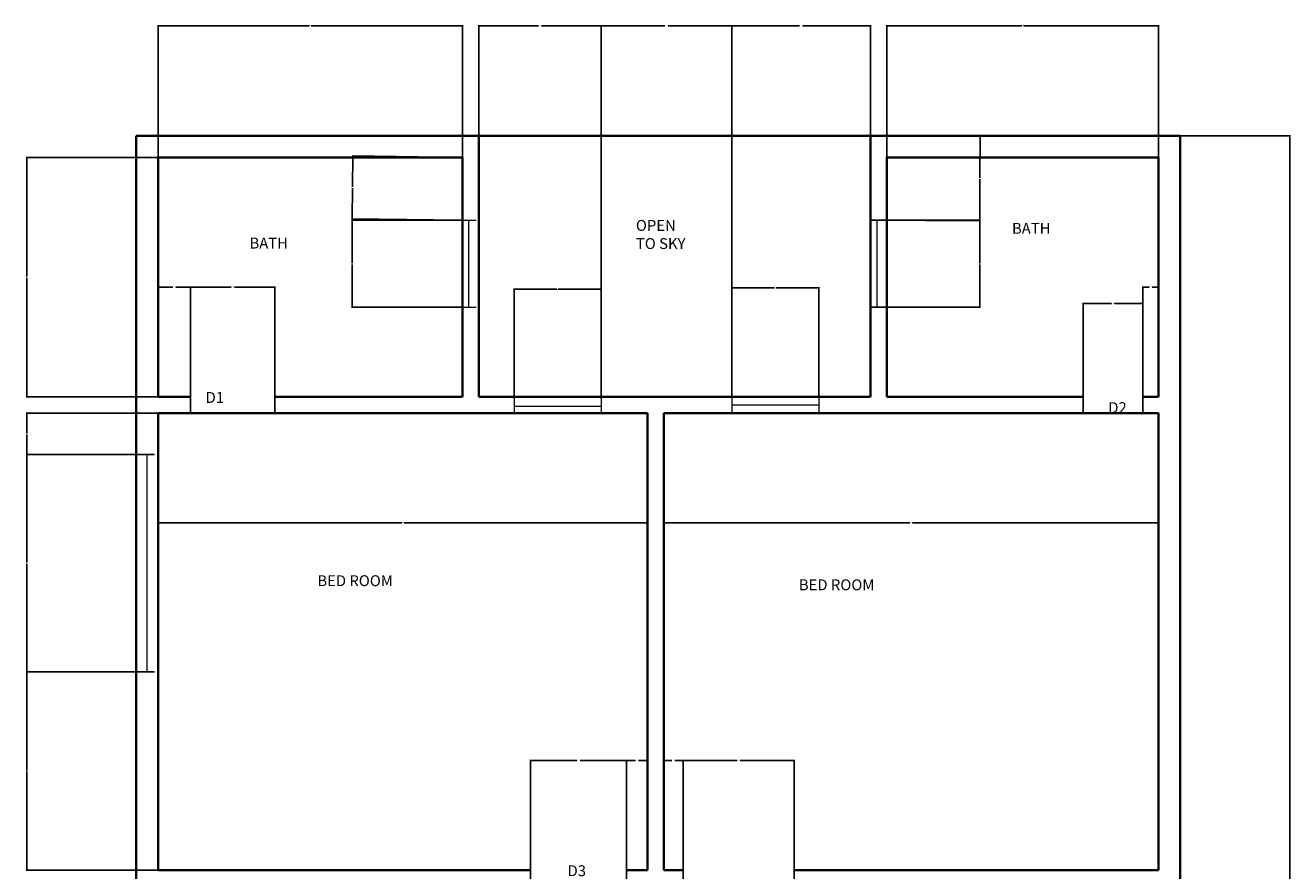
# Model space of a CAD drawing. Units: inches. Extents: x 301 to 1174, y -458 to 167.
# Tile 4 of 4: x 825 to 1174, y -66 to 167. Entities that reach past the tile are written whole.
import ezdxf

# ---------------------------------------------------------------- set-up
doc = ezdxf.new("R2010")
doc.units = ezdxf.units.IN
doc.header["$MEASUREMENT"] = 0
for name, color, linetype, lineweight in [('A-ANNO-DIMS', 2, 'Continuous', 18), ('A-ANNO-TEXT', 7, 'Continuous', 25), ('A-AREA-IDEN', 7, 'Continuous', 18), ('A-DOOR', 3, 'Continuous', 25), ('A-GLAZ', 4, 'Continuous', 18), ('A-WALL', 7, 'Continuous', 35)]:
    doc.layers.add(name, color=color, linetype=linetype, lineweight=lineweight)
doc.styles.get("Standard").update_dxf_attribs({"font": 'arial.ttf'})
doc.dimstyles.get("Standard").update_dxf_attribs({"dimtxt": 0.18, "dimasz": 0.18, "dimexe": 0.18, "dimexo": 0.0625, "dimgap": 0.09, "dimtad": 0, "dimtih": 1, "dimtoh": 1, "dimdec": 4, "dimzin": 0, "dimdsep": 46, "dimtxsty": 'Standard', "dimcen": 0.09, "dimadec": 0, "dimazin": 0, "dimtfac": 1, "dimtdec": 4, "dimtofl": 0, "dimtmove": 0, "dimatfit": 3, "dimfxl": 1, "dimtolj": 1, "dimtzin": 0, "dimarcsym": 0})

# ---------------------------------------------------------------- blocks, each defined once
blk = doc.blocks.new('*U2')
for p, q in [((0, 4), (0, 0)), ((24, 4), (24, 0)), ((0, 2), (24, 2))]:
    blk.add_line(p, q)
blk = doc.blocks.new('*U4')
for p, q in [((0, 4), (0, 0)), ((60, 4), (60, 0)), ((0, 2), (60, 2))]:
    blk.add_line(p, q)
blk = doc.blocks.new('*D39')
at = {"layer": 'A-ANNO-DIMS', "color": 0, "lineweight": -2, "transparency": 16777216}
for p, q in [((1143.26, 136.8), (1173.63, 136.8)), ((1173.45, 136.62), (1173.45, -133.02)), ((1173.45, -403.02), (1173.45, -133.38)), ((1143.26, -403.2), (1173.63, -403.2))]:
    blk.add_line(p, q, dxfattribs=at)
at = {"layer": 'A-ANNO-DIMS', "color": 0, "transparency": 16777216}
for points in [[(1173.42, 136.62), (1173.48, 136.62), (1173.45, 136.8)], [(1173.42, -403.02), (1173.48, -403.02), (1173.45, -403.2)]]:
    blk.add_solid(points, dxfattribs=at)
at = {"layer": 'Defpoints', "color": 0, "transparency": 16777216}
for p in [(1143.2, 136.8), (1173.45, 136.8), (1143.2, -403.2)]:
    blk.add_point(p, dxfattribs=at)
at = {"layer": 'A-ANNO-DIMS', "color": 0, "transparency": 16777216, "insert": (1173.45, -133.2), "char_height": 0.18, "attachment_point": 5}
blk.add_mtext('\\A1;540', dxfattribs=at)
blk = doc.blocks.new('*D40')
at = {"layer": 'A-ANNO-DIMS', "color": 0, "lineweight": -2, "transparency": 16777216}
for p, q in [((861.2, 130.86), (861.2, 167.23)), ((861.38, 167.05), (902.98, 167.05)), ((945.02, 167.05), (903.42, 167.05)), ((945.2, 130.86), (945.2, 167.23))]:
    blk.add_line(p, q, dxfattribs=at)
at = {"layer": 'A-ANNO-DIMS', "color": 0, "transparency": 16777216}
for points in [[(861.38, 167.08), (861.38, 167.02), (861.2, 167.05)], [(945.02, 167.08), (945.02, 167.02), (945.2, 167.05)]]:
    blk.add_solid(points, dxfattribs=at)
at = {"layer": 'Defpoints', "color": 0, "transparency": 16777216}
for p in [(945.2, 167.05), (861.2, 130.8), (945.2, 130.8)]:
    blk.add_point(p, dxfattribs=at)
at = {"layer": 'A-ANNO-DIMS', "color": 0, "transparency": 16777216, "insert": (903.2, 167.05), "char_height": 0.18, "attachment_point": 5}
blk.add_mtext('\\A1;84', dxfattribs=at)
blk = doc.blocks.new('*D41')
at = {"layer": 'A-ANNO-DIMS', "color": 0, "lineweight": -2, "transparency": 16777216}
for p, q in [((949.7, 136.86), (949.7, 167.23)), ((949.88, 167.05), (966.15, 167.05)), ((983.21, 167.05), (966.94, 167.05)), ((983.39, 64.27), (983.39, 167.23))]:
    blk.add_line(p, q, dxfattribs=at)
at = {"layer": 'A-ANNO-DIMS', "color": 0, "transparency": 16777216}
for points in [[(949.88, 167.08), (949.88, 167.02), (949.7, 167.05)], [(983.21, 167.08), (983.21, 167.02), (983.39, 167.05)]]:
    blk.add_solid(points, dxfattribs=at)
at = {"layer": 'Defpoints', "color": 0, "transparency": 16777216}
for p in [(983.39, 167.05), (949.7, 136.8), (983.39, 64.21)]:
    blk.add_point(p, dxfattribs=at)
at = {"layer": 'A-ANNO-DIMS', "color": 0, "transparency": 16777216, "insert": (966.54, 167.05), "char_height": 0.18, "attachment_point": 5}
blk.add_mtext('\\A1;33.69', dxfattribs=at)
blk = doc.blocks.new('*D42')
at = {"layer": 'A-ANNO-DIMS', "color": 0, "lineweight": -2, "transparency": 16777216}
for p, q in [((983.39, 64.27), (983.39, 167.23)), ((983.57, 167.05), (1000.97, 167.05)), ((1019.29, 167.05), (1001.89, 167.05)), ((1019.47, 64.65), (1019.47, 167.23))]:
    blk.add_line(p, q, dxfattribs=at)
at = {"layer": 'A-ANNO-DIMS', "color": 0, "transparency": 16777216}
for points in [[(983.57, 167.08), (983.57, 167.02), (983.39, 167.05)], [(1019.29, 167.08), (1019.29, 167.02), (1019.47, 167.05)]]:
    blk.add_solid(points, dxfattribs=at)
at = {"layer": 'Defpoints', "color": 0, "transparency": 16777216}
for p in [(1019.47, 167.05), (983.39, 64.21), (1019.47, 64.59)]:
    blk.add_point(p, dxfattribs=at)
at = {"layer": 'A-ANNO-DIMS', "color": 0, "transparency": 16777216, "insert": (1001.43, 167.05), "char_height": 0.18, "attachment_point": 5}
blk.add_mtext('\\A1;36.086', dxfattribs=at)
blk = doc.blocks.new('*D43')
at = {"layer": 'A-ANNO-DIMS', "color": 0, "lineweight": -2, "transparency": 16777216}
for p, q in [((1019.47, 64.65), (1019.47, 167.23)), ((1019.65, 167.05), (1038.19, 167.05)), ((1057.52, 167.05), (1038.98, 167.05)), ((1057.7, 136.86), (1057.7, 167.23))]:
    blk.add_line(p, q, dxfattribs=at)
at = {"layer": 'A-ANNO-DIMS', "color": 0, "transparency": 16777216}
for points in [[(1019.65, 167.08), (1019.65, 167.02), (1019.47, 167.05)], [(1057.52, 167.08), (1057.52, 167.02), (1057.7, 167.05)]]:
    blk.add_solid(points, dxfattribs=at)
at = {"layer": 'Defpoints', "color": 0, "transparency": 16777216}
for p in [(1057.7, 167.05), (1057.7, 136.8), (1019.47, 64.59)]:
    blk.add_point(p, dxfattribs=at)
at = {"layer": 'A-ANNO-DIMS', "color": 0, "transparency": 16777216, "insert": (1038.59, 167.05), "char_height": 0.18, "attachment_point": 5}
blk.add_mtext('\\A1;38.22', dxfattribs=at)
blk = doc.blocks.new('*D44')
at = {"layer": 'A-ANNO-DIMS', "color": 0, "lineweight": -2, "transparency": 16777216}
for p, q in [((1062.2, 130.86), (1062.2, 167.23)), ((1062.38, 167.05), (1099.48, 167.05)), ((1137.02, 167.05), (1099.92, 167.05)), ((1137.2, 130.86), (1137.2, 167.23))]:
    blk.add_line(p, q, dxfattribs=at)
at = {"layer": 'A-ANNO-DIMS', "color": 0, "transparency": 16777216}
for points in [[(1062.38, 167.08), (1062.38, 167.02), (1062.2, 167.05)], [(1137.02, 167.08), (1137.02, 167.02), (1137.2, 167.05)]]:
    blk.add_solid(points, dxfattribs=at)
at = {"layer": 'Defpoints', "color": 0, "transparency": 16777216}
for p in [(1137.2, 167.05), (1062.2, 130.8), (1137.2, 130.8)]:
    blk.add_point(p, dxfattribs=at)
at = {"layer": 'A-ANNO-DIMS', "color": 0, "transparency": 16777216, "insert": (1099.7, 167.05), "char_height": 0.18, "attachment_point": 5}
blk.add_mtext('\\A1;75', dxfattribs=at)
blk = doc.blocks.new('*D45')
at = {"layer": 'A-ANNO-DIMS', "color": 0, "lineweight": -2, "transparency": 16777216}
for p, q in [((959.39, 64.27), (959.39, 94.64)), ((959.57, 94.46), (971.17, 94.46)), ((983.21, 94.46), (971.61, 94.46)), ((983.39, 64.27), (983.39, 94.64))]:
    blk.add_line(p, q, dxfattribs=at)
at = {"layer": 'A-ANNO-DIMS', "color": 0, "transparency": 16777216}
for points in [[(959.57, 94.49), (959.57, 94.43), (959.39, 94.46)], [(983.21, 94.49), (983.21, 94.43), (983.39, 94.46)]]:
    blk.add_solid(points, dxfattribs=at)
at = {"layer": 'Defpoints', "color": 0, "transparency": 16777216}
for p in [(983.39, 94.46), (959.39, 64.21), (983.39, 64.21)]:
    blk.add_point(p, dxfattribs=at)
at = {"layer": 'A-ANNO-DIMS', "color": 0, "transparency": 16777216, "insert": (971.39, 94.46), "char_height": 0.18, "attachment_point": 5}
blk.add_mtext('\\A1;24', dxfattribs=at)
blk = doc.blocks.new('*D46')
at = {"layer": 'A-ANNO-DIMS', "color": 0, "lineweight": -2, "transparency": 16777216}
for p, q in [((1019.47, 64.65), (1019.47, 95.02)), ((1019.65, 94.84), (1031.25, 94.84)), ((1043.29, 94.84), (1031.69, 94.84)), ((1043.47, 64.65), (1043.47, 95.02))]:
    blk.add_line(p, q, dxfattribs=at)
at = {"layer": 'A-ANNO-DIMS', "color": 0, "transparency": 16777216}
for points in [[(1019.65, 94.87), (1019.65, 94.81), (1019.47, 94.84)], [(1043.29, 94.87), (1043.29, 94.81), (1043.47, 94.84)]]:
    blk.add_solid(points, dxfattribs=at)
at = {"layer": 'Defpoints', "color": 0, "transparency": 16777216}
for p in [(1043.47, 94.84), (1019.47, 64.59), (1043.47, 64.59)]:
    blk.add_point(p, dxfattribs=at)
at = {"layer": 'A-ANNO-DIMS', "color": 0, "transparency": 16777216, "insert": (1031.47, 94.84), "char_height": 0.18, "attachment_point": 5}
blk.add_mtext('\\A1;24', dxfattribs=at)
blk = doc.blocks.new('*D47')
at = {"layer": 'A-ANNO-DIMS', "color": 0, "lineweight": -2, "transparency": 16777216}
for p, q in [((861.2, 60.24), (861.2, 29.87)), ((996.2, 60.24), (996.2, 29.87)), ((861.38, 30.05), (928.42, 30.05)), ((996.02, 30.05), (928.98, 30.05))]:
    blk.add_line(p, q, dxfattribs=at)
at = {"layer": 'A-ANNO-DIMS', "color": 0, "transparency": 16777216}
for points in [[(861.38, 30.08), (861.38, 30.02), (861.2, 30.05)], [(996.02, 30.08), (996.02, 30.02), (996.2, 30.05)]]:
    blk.add_solid(points, dxfattribs=at)
at = {"layer": 'Defpoints', "color": 0, "transparency": 16777216}
for p in [(861.2, 60.3), (996.2, 60.3), (861.2, 30.05)]:
    blk.add_point(p, dxfattribs=at)
at = {"layer": 'A-ANNO-DIMS', "color": 0, "transparency": 16777216, "insert": (928.7, 30.05), "char_height": 0.18, "attachment_point": 5}
blk.add_mtext('\\A1;135', dxfattribs=at)
blk = doc.blocks.new('*D48')
at = {"layer": 'A-ANNO-DIMS', "color": 0, "lineweight": -2, "transparency": 16777216}
for p, q in [((1000.7, 60.24), (1000.7, 29.87)), ((1137.2, 60.24), (1137.2, 29.87)), ((1000.88, 30.05), (1068.56, 30.05)), ((1137.02, 30.05), (1069.33, 30.05))]:
    blk.add_line(p, q, dxfattribs=at)
at = {"layer": 'A-ANNO-DIMS', "color": 0, "transparency": 16777216}
for points in [[(1000.88, 30.08), (1000.88, 30.02), (1000.7, 30.05)], [(1137.02, 30.08), (1137.02, 30.02), (1137.2, 30.05)]]:
    blk.add_solid(points, dxfattribs=at)
at = {"layer": 'Defpoints', "color": 0, "transparency": 16777216}
for p in [(1000.7, 60.3), (1137.2, 60.3), (1000.7, 30.05)]:
    blk.add_point(p, dxfattribs=at)
at = {"layer": 'A-ANNO-DIMS', "color": 0, "transparency": 16777216, "insert": (1068.95, 30.05), "char_height": 0.18, "attachment_point": 5}
blk.add_mtext('\\A1;136.5', dxfattribs=at)
blk = doc.blocks.new('*D55')
at = {"layer": 'A-ANNO-DIMS', "color": 0, "lineweight": -2, "transparency": 16777216}
for p, q in [((861.13, 130.8), (824.77, 130.8)), ((824.95, 130.62), (824.95, 97.98)), ((824.95, 64.98), (824.95, 97.62)), ((861.13, 64.8), (824.77, 64.8))]:
    blk.add_line(p, q, dxfattribs=at)
at = {"layer": 'A-ANNO-DIMS', "color": 0, "transparency": 16777216}
for points in [[(824.92, 130.62), (824.98, 130.62), (824.95, 130.8)], [(824.92, 64.98), (824.98, 64.98), (824.95, 64.8)]]:
    blk.add_solid(points, dxfattribs=at)
at = {"layer": 'Defpoints', "color": 0, "transparency": 16777216}
for p in [(824.95, 130.8), (861.2, 130.8), (861.2, 64.8)]:
    blk.add_point(p, dxfattribs=at)
at = {"layer": 'A-ANNO-DIMS', "color": 0, "transparency": 16777216, "insert": (824.95, 97.8), "char_height": 0.18, "attachment_point": 5}
blk.add_mtext('\\A1;66', dxfattribs=at)
blk = doc.blocks.new('*D56')
at = {"layer": 'A-ANNO-DIMS', "color": 0, "lineweight": -2, "transparency": 16777216}
for p, q in [((860.11, -11.08), (824.77, -11.08)), ((824.95, -11.26), (824.95, -38.21)), ((824.95, -65.52), (824.95, -38.57)), ((861.13, -65.7), (824.77, -65.7))]:
    blk.add_line(p, q, dxfattribs=at)
at = {"layer": 'A-ANNO-DIMS', "color": 0, "transparency": 16777216}
for points in [[(824.92, -11.26), (824.98, -11.26), (824.95, -11.08)], [(824.92, -65.52), (824.98, -65.52), (824.95, -65.7)]]:
    blk.add_solid(points, dxfattribs=at)
at = {"layer": 'Defpoints', "color": 0, "transparency": 16777216}
for p in [(824.95, -11.08), (860.17, -11.08), (861.2, -65.7)]:
    blk.add_point(p, dxfattribs=at)
at = {"layer": 'A-ANNO-DIMS', "color": 0, "transparency": 16777216, "insert": (824.95, -38.39), "char_height": 0.18, "attachment_point": 5}
blk.add_mtext('\\A1;54.61', dxfattribs=at)
blk = doc.blocks.new('*D57')
at = {"layer": 'A-ANNO-DIMS', "color": 0, "lineweight": -2, "transparency": 16777216}
for p, q in [((860.11, 48.92), (824.77, 48.92)), ((824.95, 48.74), (824.95, 19.1)), ((824.95, -10.9), (824.95, 18.73)), ((860.11, -11.08), (824.77, -11.08))]:
    blk.add_line(p, q, dxfattribs=at)
at = {"layer": 'A-ANNO-DIMS', "color": 0, "transparency": 16777216}
for points in [[(824.92, 48.74), (824.98, 48.74), (824.95, 48.92)], [(824.92, -10.9), (824.98, -10.9), (824.95, -11.08)]]:
    blk.add_solid(points, dxfattribs=at)
at = {"layer": 'Defpoints', "color": 0, "transparency": 16777216}
for p in [(824.95, 48.92), (860.17, 48.92), (860.17, -11.08)]:
    blk.add_point(p, dxfattribs=at)
at = {"layer": 'A-ANNO-DIMS', "color": 0, "transparency": 16777216, "insert": (824.95, 18.92), "char_height": 0.18, "attachment_point": 5}
blk.add_mtext('\\A1;60', dxfattribs=at)
blk = doc.blocks.new('*D58')
at = {"layer": 'A-ANNO-DIMS', "color": 0, "lineweight": -2, "transparency": 16777216}
for p, q in [((861.13, 60.3), (824.77, 60.3)), ((824.95, 60.12), (824.95, 54.79)), ((824.95, 49.1), (824.95, 54.43)), ((860.11, 48.92), (824.77, 48.92))]:
    blk.add_line(p, q, dxfattribs=at)
at = {"layer": 'A-ANNO-DIMS', "color": 0, "transparency": 16777216}
for points in [[(824.92, 60.12), (824.98, 60.12), (824.95, 60.3)], [(824.92, 49.1), (824.98, 49.1), (824.95, 48.92)]]:
    blk.add_solid(points, dxfattribs=at)
at = {"layer": 'Defpoints', "color": 0, "transparency": 16777216}
for p in [(824.95, 60.3), (861.2, 60.3), (860.17, 48.92)]:
    blk.add_point(p, dxfattribs=at)
at = {"layer": 'A-ANNO-DIMS', "color": 0, "transparency": 16777216, "insert": (824.95, 54.61), "char_height": 0.18, "attachment_point": 5}
blk.add_mtext('\\A1;11.386', dxfattribs=at)
blk = doc.blocks.new('*D66')
at = {"layer": 'A-ANNO-DIMS', "color": 0, "lineweight": -2, "transparency": 16777216}
for p, q in [((861.2, 64.86), (861.2, 95.23)), ((861.38, 95.05), (865.29, 95.05)), ((869.98, 95.05), (866.07, 95.05)), ((870.16, 64.86), (870.16, 95.23))]:
    blk.add_line(p, q, dxfattribs=at)
at = {"layer": 'A-ANNO-DIMS', "color": 0, "transparency": 16777216}
for points in [[(861.38, 95.08), (861.38, 95.02), (861.2, 95.05)], [(869.98, 95.08), (869.98, 95.02), (870.16, 95.05)]]:
    blk.add_solid(points, dxfattribs=at)
at = {"layer": 'Defpoints', "color": 0, "transparency": 16777216}
for p in [(870.16, 95.05), (861.2, 64.8), (870.16, 64.8)]:
    blk.add_point(p, dxfattribs=at)
at = {"layer": 'A-ANNO-DIMS', "color": 0, "transparency": 16777216, "insert": (865.68, 95.05), "char_height": 0.18, "attachment_point": 5}
blk.add_mtext('\\A1;8.962', dxfattribs=at)
blk = doc.blocks.new('*D67')
at = {"layer": 'A-ANNO-DIMS', "color": 0, "lineweight": -2, "transparency": 16777216}
for p, q in [((870.16, 64.86), (870.16, 95.23)), ((870.34, 95.05), (881.33, 95.05)), ((893.25, 95.05), (882.26, 95.05)), ((893.43, 64.86), (893.43, 95.23))]:
    blk.add_line(p, q, dxfattribs=at)
at = {"layer": 'A-ANNO-DIMS', "color": 0, "transparency": 16777216}
for points in [[(870.34, 95.08), (870.34, 95.02), (870.16, 95.05)], [(893.25, 95.08), (893.25, 95.02), (893.43, 95.05)]]:
    blk.add_solid(points, dxfattribs=at)
at = {"layer": 'Defpoints', "color": 0, "transparency": 16777216}
for p in [(893.43, 95.05), (870.16, 64.8), (893.43, 64.8)]:
    blk.add_point(p, dxfattribs=at)
at = {"layer": 'A-ANNO-DIMS', "color": 0, "transparency": 16777216, "insert": (881.79, 95.05), "char_height": 0.18, "attachment_point": 5}
blk.add_mtext('\\A1;23.267', dxfattribs=at)
blk = doc.blocks.new('*D68')
at = {"layer": 'A-ANNO-DIMS', "color": 0, "lineweight": -2, "transparency": 16777216}
for p, q in [((1116.42, 60.36), (1116.42, 90.73)), ((1116.6, 90.55), (1124.18, 90.55)), ((1132.68, 90.55), (1125.09, 90.55)), ((1132.86, 60.36), (1132.86, 90.73))]:
    blk.add_line(p, q, dxfattribs=at)
at = {"layer": 'A-ANNO-DIMS', "color": 0, "transparency": 16777216}
for points in [[(1116.6, 90.58), (1116.6, 90.52), (1116.42, 90.55)], [(1132.68, 90.58), (1132.68, 90.52), (1132.86, 90.55)]]:
    blk.add_solid(points, dxfattribs=at)
at = {"layer": 'Defpoints', "color": 0, "transparency": 16777216}
for p in [(1132.86, 90.55), (1116.42, 60.3), (1132.86, 60.3)]:
    blk.add_point(p, dxfattribs=at)
at = {"layer": 'A-ANNO-DIMS', "color": 0, "transparency": 16777216, "insert": (1124.64, 90.55), "char_height": 0.18, "attachment_point": 5}
blk.add_mtext('\\A1;16.434', dxfattribs=at)
blk = doc.blocks.new('*D69')
at = {"layer": 'A-ANNO-DIMS', "color": 0, "lineweight": -2, "transparency": 16777216}
for p, q in [((1132.86, 64.86), (1132.86, 95.23)), ((1133.04, 95.05), (1134.63, 95.05)), ((1137.02, 95.05), (1135.42, 95.05)), ((1137.2, 64.86), (1137.2, 95.23))]:
    blk.add_line(p, q, dxfattribs=at)
at = {"layer": 'A-ANNO-DIMS', "color": 0, "transparency": 16777216}
for points in [[(1133.04, 95.08), (1133.04, 95.02), (1132.86, 95.05)], [(1137.02, 95.08), (1137.02, 95.02), (1137.2, 95.05)]]:
    blk.add_solid(points, dxfattribs=at)
at = {"layer": 'Defpoints', "color": 0, "transparency": 16777216}
for p in [(1137.2, 95.05), (1132.86, 64.8), (1137.2, 64.8)]:
    blk.add_point(p, dxfattribs=at)
at = {"layer": 'A-ANNO-DIMS', "color": 0, "transparency": 16777216, "insert": (1135.03, 95.05), "char_height": 0.18, "attachment_point": 5}
blk.add_mtext('\\A1;4.342', dxfattribs=at)
blk = doc.blocks.new('*D70')
at = {"layer": 'A-ANNO-DIMS', "color": 0, "lineweight": -2, "transparency": 16777216}
for p, q in [((944.9, 113.47), (914.54, 113.47)), ((914.72, 113.29), (914.72, 101.65)), ((914.72, 89.65), (914.72, 101.29)), ((944.9, 89.47), (914.54, 89.47))]:
    blk.add_line(p, q, dxfattribs=at)
at = {"layer": 'A-ANNO-DIMS', "color": 0, "transparency": 16777216}
for points in [[(914.69, 113.29), (914.75, 113.29), (914.72, 113.47)], [(914.69, 89.65), (914.75, 89.65), (914.72, 89.47)]]:
    blk.add_solid(points, dxfattribs=at)
at = {"layer": 'Defpoints', "color": 0, "transparency": 16777216}
for p in [(914.72, 113.47), (944.97, 113.47), (944.97, 89.47)]:
    blk.add_point(p, dxfattribs=at)
at = {"layer": 'A-ANNO-DIMS', "color": 0, "transparency": 16777216, "insert": (914.72, 101.47), "char_height": 0.18, "attachment_point": 5}
blk.add_mtext('\\A1;24', dxfattribs=at)
blk = doc.blocks.new('*D71')
at = {"layer": 'A-ANNO-DIMS', "color": 0, "lineweight": -2, "transparency": 16777216}
for p, q in [((945.13, 130.8), (914.77, 131.21)), ((914.95, 131.02), (914.84, 122.72)), ((914.72, 114.05), (914.83, 122.36)), ((944.9, 113.47), (914.54, 113.87))]:
    blk.add_line(p, q, dxfattribs=at)
at = {"layer": 'A-ANNO-DIMS', "color": 0, "transparency": 16777216}
for points in [[(914.92, 131.02), (914.98, 131.02), (914.95, 131.2)], [(914.69, 114.05), (914.75, 114.05), (914.72, 113.87)]]:
    blk.add_solid(points, dxfattribs=at)
at = {"layer": 'Defpoints', "color": 0, "transparency": 16777216}
for p in [(914.95, 131.2), (945.2, 130.8), (944.97, 113.47)]:
    blk.add_point(p, dxfattribs=at)
at = {"layer": 'A-ANNO-DIMS', "color": 0, "transparency": 16777216, "insert": (914.83, 122.54), "char_height": 0.18, "attachment_point": 5}
blk.add_mtext('\\A1;17.334', dxfattribs=at)
blk = doc.blocks.new('*D72')
at = {"layer": 'A-ANNO-DIMS', "color": 0, "lineweight": -2, "transparency": 16777216}
for p, q in [((1057.76, 136.8), (1088.13, 136.69)), ((1087.95, 136.51), (1087.9, 125.2)), ((1087.86, 113.54), (1087.9, 124.84)), ((1057.67, 113.47), (1088.04, 113.36))]:
    blk.add_line(p, q, dxfattribs=at)
at = {"layer": 'A-ANNO-DIMS', "color": 0, "transparency": 16777216}
for points in [[(1087.92, 136.51), (1087.98, 136.51), (1087.95, 136.69)], [(1087.83, 113.54), (1087.89, 113.54), (1087.86, 113.36)]]:
    blk.add_solid(points, dxfattribs=at)
at = {"layer": 'Defpoints', "color": 0, "transparency": 16777216}
for p in [(1057.7, 136.8), (1057.61, 113.47), (1087.86, 113.36)]:
    blk.add_point(p, dxfattribs=at)
at = {"layer": 'A-ANNO-DIMS', "color": 0, "transparency": 16777216, "insert": (1087.9, 125.02), "char_height": 0.18, "attachment_point": 5}
blk.add_mtext('\\A1;23.33', dxfattribs=at)
blk = doc.blocks.new('*D73')
at = {"layer": 'A-ANNO-DIMS', "color": 0, "lineweight": -2, "transparency": 16777216}
for p, q in [((1057.67, 113.47), (1088.04, 113.47)), ((1087.86, 113.29), (1087.86, 101.65)), ((1087.86, 89.65), (1087.86, 101.29)), ((1057.67, 89.47), (1088.04, 89.47))]:
    blk.add_line(p, q, dxfattribs=at)
at = {"layer": 'A-ANNO-DIMS', "color": 0, "transparency": 16777216}
for points in [[(1087.83, 113.29), (1087.89, 113.29), (1087.86, 113.47)], [(1087.83, 89.65), (1087.89, 89.65), (1087.86, 89.47)]]:
    blk.add_solid(points, dxfattribs=at)
at = {"layer": 'Defpoints', "color": 0, "transparency": 16777216}
for p in [(1057.61, 113.47), (1057.61, 89.47), (1087.86, 89.47)]:
    blk.add_point(p, dxfattribs=at)
at = {"layer": 'A-ANNO-DIMS', "color": 0, "transparency": 16777216, "insert": (1087.86, 101.47), "char_height": 0.18, "attachment_point": 5}
blk.add_mtext('\\A1;24', dxfattribs=at)
blk = doc.blocks.new('*D74')
at = {"layer": 'A-ANNO-DIMS', "color": 0, "lineweight": -2, "transparency": 16777216}
for p, q in [((963.97, -65.64), (963.97, -35.27)), ((964.15, -35.45), (976.74, -35.45)), ((990.26, -35.45), (977.67, -35.45)), ((990.44, -65.64), (990.44, -35.27))]:
    blk.add_line(p, q, dxfattribs=at)
at = {"layer": 'A-ANNO-DIMS', "color": 0, "transparency": 16777216}
for points in [[(964.15, -35.42), (964.15, -35.48), (963.97, -35.45)], [(990.26, -35.42), (990.26, -35.48), (990.44, -35.45)]]:
    blk.add_solid(points, dxfattribs=at)
at = {"layer": 'Defpoints', "color": 0, "transparency": 16777216}
for p in [(990.44, -35.45), (963.97, -65.7), (990.44, -65.7)]:
    blk.add_point(p, dxfattribs=at)
at = {"layer": 'A-ANNO-DIMS', "color": 0, "transparency": 16777216, "insert": (977.2, -35.45), "char_height": 0.18, "attachment_point": 5}
blk.add_mtext('\\A1;26.474', dxfattribs=at)
blk = doc.blocks.new('*D75')
at = {"layer": 'A-ANNO-DIMS', "color": 0, "lineweight": -2, "transparency": 16777216}
for p, q in [((990.44, -65.64), (990.44, -35.27)), ((990.62, -35.45), (992.92, -35.45)), ((996.02, -35.45), (993.71, -35.45)), ((996.2, -65.64), (996.2, -35.27))]:
    blk.add_line(p, q, dxfattribs=at)
at = {"layer": 'A-ANNO-DIMS', "color": 0, "transparency": 16777216}
for points in [[(990.62, -35.42), (990.62, -35.48), (990.44, -35.45)], [(996.02, -35.42), (996.02, -35.48), (996.2, -35.45)]]:
    blk.add_solid(points, dxfattribs=at)
at = {"layer": 'Defpoints', "color": 0, "transparency": 16777216}
for p in [(996.2, -35.45), (990.44, -65.7), (996.2, -65.7)]:
    blk.add_point(p, dxfattribs=at)
at = {"layer": 'A-ANNO-DIMS', "color": 0, "transparency": 16777216, "insert": (993.32, -35.45), "char_height": 0.18, "attachment_point": 5}
blk.add_mtext('\\A1;5.758', dxfattribs=at)
blk = doc.blocks.new('*D76')
at = {"layer": 'A-ANNO-DIMS', "color": 0, "lineweight": -2, "transparency": 16777216}
for p, q in [((1000.7, -65.64), (1000.7, -35.27)), ((1000.88, -35.45), (1002.96, -35.45)), ((1005.84, -35.45), (1003.75, -35.45)), ((1006.02, -65.64), (1006.02, -35.27))]:
    blk.add_line(p, q, dxfattribs=at)
at = {"layer": 'A-ANNO-DIMS', "color": 0, "transparency": 16777216}
for points in [[(1000.88, -35.42), (1000.88, -35.48), (1000.7, -35.45)], [(1005.84, -35.42), (1005.84, -35.48), (1006.02, -35.45)]]:
    blk.add_solid(points, dxfattribs=at)
at = {"layer": 'Defpoints', "color": 0, "transparency": 16777216}
for p in [(1006.02, -35.45), (1000.7, -65.7), (1006.02, -65.7)]:
    blk.add_point(p, dxfattribs=at)
at = {"layer": 'A-ANNO-DIMS', "color": 0, "transparency": 16777216, "insert": (1003.36, -35.45), "char_height": 0.18, "attachment_point": 5}
blk.add_mtext('\\A1;5.319', dxfattribs=at)
blk = doc.blocks.new('*D77')
at = {"layer": 'A-ANNO-DIMS', "color": 0, "lineweight": -2, "transparency": 16777216}
for p, q in [((1006.02, -65.64), (1006.02, -35.27)), ((1006.2, -35.45), (1020.96, -35.45)), ((1036.52, -35.45), (1021.75, -35.45)), ((1036.7, -65.64), (1036.7, -35.27))]:
    blk.add_line(p, q, dxfattribs=at)
at = {"layer": 'A-ANNO-DIMS', "color": 0, "transparency": 16777216}
for points in [[(1006.2, -35.42), (1006.2, -35.48), (1006.02, -35.45)], [(1036.52, -35.42), (1036.52, -35.48), (1036.7, -35.45)]]:
    blk.add_solid(points, dxfattribs=at)
at = {"layer": 'Defpoints', "color": 0, "transparency": 16777216}
for p in [(1036.7, -35.45), (1006.02, -65.7), (1036.7, -65.7)]:
    blk.add_point(p, dxfattribs=at)
at = {"layer": 'A-ANNO-DIMS', "color": 0, "transparency": 16777216, "insert": (1021.36, -35.45), "char_height": 0.18, "attachment_point": 5}
blk.add_mtext('\\A1;30.68', dxfattribs=at)

msp = doc.modelspace()

# ---------------------------------------------------------------- linework, layer by layer
at = {"layer": 'A-DOOR'}
for p, q in [((870.1592, 64.8013), (870.1592, 60.3013)), ((893.4265, 64.8013), (893.4265, 64.8013)), ((893.4265, 64.8013), (893.4265, 60.3013)), ((1116.4216, 64.8013), (1116.4216, 60.3013)), ((1132.8555, 64.8013), (1132.8555, 60.3013)), ((963.9661, -65.6987), (963.9661, -70.1987)), ((990.4397, -65.6987), (990.4397, -70.1987)), ((1006.0166, -65.6987), (1006.0166, -70.1987)), ((1036.6974, -70.1987), (1036.6974, -65.6987))]:
    msp.add_line(p, q, dxfattribs=at)
at = {"layer": 'A-WALL'}
for p, q in [((855.1974, 136.8013), (1143.1974, 136.8013)), ((855.1974, -403.1987), (855.1974, 136.8013)), ((949.6974, 130.8013), (949.6974, 136.8013)), ((1057.6974, 130.8013), (1057.6974, 136.8013)), ((1143.1974, 136.8013), (1143.1974, -403.1987)), ((861.1974, 130.8013), (945.1974, 130.8013)), ((861.1974, 64.8013), (861.1974, 130.8013)), ((945.1974, 130.8013), (945.1974, 64.8013)), ((949.6974, 130.8013), (949.6974, 64.8013)), ((1057.6974, 64.8013), (1057.6974, 130.8013)), ((1057.6974, 130.8013), (1057.6974, 130.8013)), ((1062.1974, 130.8013), (1137.1974, 130.8013)), ((1062.1974, 64.8013), (1062.1974, 130.8013)), ((1137.1974, 130.8013), (1137.1974, 64.8013)), ((870.1592, 64.8013), (861.1974, 64.8013)), ((945.1974, 64.8013), (893.4265, 64.8013)), ((949.6974, 64.8013), (1057.6974, 64.8013)), ((1062.1974, 64.8013), (1116.4216, 64.8013)), ((1132.8555, 64.8013), (1137.1974, 64.8013)), ((861.1974, -65.6987), (861.1974, 60.3013)), ((945.1974, 60.3013), (861.1974, 60.3013)), ((861.1974, 60.3013), (861.1974, -65.6987)), ((945.1974, 60.3013), (949.6974, 60.3013)), ((949.6974, 60.3013), (996.1974, 60.3013)), ((996.1974, -65.6987), (996.1974, 60.3013)), ((1000.6974, 60.3013), (1057.6974, 60.3013)), ((1000.6974, -65.6987), (1000.6974, 60.3013)), ((1057.6974, 60.3013), (1062.2265, 60.3013)), ((1062.1974, 60.3013), (1137.1974, 60.3013)), ((1137.1974, 60.3013), (1137.1974, -65.6987)), ((861.1974, -65.6987), (963.9661, -65.6987)), ((990.4397, -65.6987), (996.1974, -65.6987)), ((1000.6974, -65.6987), (1006.0166, -65.6987)), ((1036.6974, -65.6987), (1137.1974, -65.6987))]:
    msp.add_line(p, q, dxfattribs=at)

# ---------------------------------------------------------------- block references
at = {"layer": 'A-GLAZ', "rotation": 90}
for name, p in [('*U2', (948.9672, 89.4692)), ('*U2', (1061.6108, 89.4692)), ('*U4', (860.17, -11.0847))]:
    msp.add_blockref(name, p, dxfattribs=at)
at = {"layer": 'A-GLAZ'}
for p in [(959.3882, 60.2056), (1019.474, 60.5865)]:
    msp.add_blockref('*U2', p, dxfattribs=at)

# ---------------------------------------------------------------- texts
at = {"layer": 'A-ANNO-TEXT', "char_height": 3, "attachment_point": 1}
for s, insert in [('D1', (874.3089, 66.1204)), ('D2', (1123.3335, 63.3136)), ('D3', (974.1661, -64.3886))]:
    msp.add_mtext_dynamic_manual_height_columns(s, width=13.351331, gutter_width=1, heights=[0], dxfattribs=dict(at, insert=insert))
at = {"layer": 'A-AREA-IDEN', "char_height": 0.2, "attachment_point": 1}
for s, insert in [('{\\H15x;OPEN\\PTO SKY}', (993.0194, 113.5518)), ('{\\H15x;BATH}', (1096.7652, 112.7388)), ('{\\H15x;BATH}', (886.4257, 108.6736)), ('{\\H15x;BED ROOM}', (905.1407, 15.5805)), ('{\\H15x;BED ROOM}', (1037.9748, 14.4515))]:
    msp.add_mtext_dynamic_manual_height_columns(s, width=70.987625, gutter_width=1, heights=[0], dxfattribs=dict(at, insert=insert))

# ---------------------------------------------------------------- dimensions: what is measured, and where the dimension line sits
at = {"layer": 'A-ANNO-DIMS'}
for base, p1, p2, override, picture, middle in [((945.1974, 167.0513), (861.1974, 130.8013), (945.1974, 130.8013), {"dimdec": 0, "dimlfac": 1, "dimrnd": 0, "dimzin": 0, "dimdsep": 46, "dimlunit": 2}, '*D40', (903.1974, 167.0513)), ((983.3882, 167.0513), (949.6974, 136.8013), (983.3882, 64.2056), {"dimdec": 2, "dimlfac": 1, "dimrnd": 0, "dimzin": 0, "dimdsep": 46, "dimlunit": 2}, '*D41', (966.5428, 167.0513)), ((1019.474, 167.0513), (983.3882, 64.2056), (1019.474, 64.5865), {"dimdec": 3, "dimlfac": 1, "dimrnd": 0, "dimzin": 0, "dimdsep": 46, "dimlunit": 2}, '*D42', (1001.4311, 167.0513)), ((1057.6974, 167.0513), (1019.474, 64.5865), (1057.6974, 136.8013), {"dimdec": 2, "dimlfac": 1, "dimrnd": 0, "dimzin": 0, "dimdsep": 46, "dimlunit": 2}, '*D43', (1038.5857, 167.0513)), ((1137.1974, 167.0513), (1062.1974, 130.8013), (1137.1974, 130.8013), {"dimdec": 0, "dimlfac": 1, "dimrnd": 0, "dimzin": 0, "dimdsep": 46, "dimlunit": 2}, '*D44', (1099.6974, 167.0513)), ((893.4265, 95.0513), (870.1592, 64.8013), (893.4265, 64.8013), {"dimdec": 3, "dimlfac": 1, "dimrnd": 0, "dimzin": 0, "dimdsep": 46, "dimlunit": 2}, '*D67', (881.7929, 95.0513)), ((983.3882, 94.4556), (959.3882, 64.2056), (983.3882, 64.2056), {"dimdec": 0, "dimlfac": 1, "dimrnd": 0, "dimzin": 0, "dimdsep": 46, "dimlunit": 2}, '*D45', (971.3882, 94.4556)), ((1043.474, 94.8365), (1019.474, 64.5865), (1043.474, 64.5865), {"dimdec": 0, "dimlfac": 1, "dimrnd": 0, "dimzin": 0, "dimdsep": 46, "dimlunit": 2}, '*D46', (1031.474, 94.8365)), ((1137.1974, 95.0513), (1132.8555, 64.8013), (1137.1974, 64.8013), {"dimdec": 3, "dimlfac": 1, "dimrnd": 0, "dimzin": 0, "dimdsep": 46, "dimlunit": 2}, '*D69', (1135.0265, 95.0513)), ((1132.8555, 90.5513), (1116.4216, 60.3013), (1132.8555, 60.3013), {"dimdec": 3, "dimlfac": 1, "dimrnd": 0, "dimzin": 0, "dimdsep": 46, "dimlunit": 2}, '*D68', (1124.6386, 90.5513)), ((990.4397, -35.4487), (963.9661, -65.6987), (990.4397, -65.6987), {"dimdec": 3, "dimlfac": 1, "dimrnd": 0, "dimzin": 0, "dimdsep": 46, "dimlunit": 2}, '*D74', (977.2029, -35.4487)), ((996.1974, -35.4487), (990.4397, -65.6987), (996.1974, -65.6987), {"dimdec": 3, "dimlfac": 1, "dimrnd": 0, "dimzin": 0, "dimdsep": 46, "dimlunit": 2}, '*D75', (993.3186, -35.4487)), ((1006.0166, -35.4487), (1000.6974, -65.6987), (1006.0166, -65.6987), {"dimdec": 3, "dimlfac": 1, "dimrnd": 0, "dimzin": 0, "dimdsep": 46, "dimlunit": 2}, '*D76', (1003.357, -35.4487))]:
    dim = msp.add_linear_dim(base=base, p1=p1, p2=p2, dimstyle='Standard', override=override, dxfattribs=at)
    dim.commit()
    dim.dimension.update_dxf_attribs({"geometry": picture, "text_midpoint": middle})
for base, p1, p2, angle, override, picture, middle in [((1087.8606, 113.3569), (1057.6974, 136.8013), (1057.6108, 113.4692), 269.787275, {"dimdec": 2, "dimlfac": 1, "dimrnd": 0, "dimzin": 0, "dimdsep": 46, "dimlunit": 2}, '*D72', (1087.9039, 125.023)), ((1173.4474, 136.8013), (1143.1974, -403.1987), (1143.1974, 136.8013), 90, {"dimdec": 0, "dimlfac": 1, "dimrnd": 0, "dimzin": 0, "dimdsep": 46, "dimlunit": 2}, '*D39', (1173.4474, -133.1987)), ((824.9474, 130.8013), (861.1974, 64.8013), (861.1974, 130.8013), 90, {"dimdec": 0, "dimlfac": 1, "dimrnd": 0, "dimzin": 0, "dimdsep": 46, "dimlunit": 2}, '*D55', (824.9474, 97.8013)), ((914.9501, 131.2032), (944.9672, 113.4692), (945.1974, 130.8013), 89.238783, {"dimdec": 3, "dimlfac": 1, "dimrnd": 0, "dimzin": 0, "dimdsep": 46, "dimlunit": 2}, '*D71', (914.835, 122.5371)), ((914.7172, 113.4692), (944.9672, 89.4692), (944.9672, 113.4692), 90, {"dimdec": 0, "dimlfac": 1, "dimrnd": 0, "dimzin": 0, "dimdsep": 46, "dimlunit": 2}, '*D70', (914.7172, 101.4692)), ((1087.8608, 89.4692), (1057.6108, 113.4692), (1057.6108, 89.4692), 270, {"dimdec": 0, "dimlfac": 1, "dimrnd": 0, "dimzin": 0, "dimdsep": 46, "dimlunit": 2}, '*D73', (1087.8608, 101.4692)), ((870.1592, 95.0513), (861.1974, 64.8013), (870.1592, 64.8013), 0, {"dimdec": 3, "dimlfac": 1, "dimrnd": 0, "dimzin": 0, "dimdsep": 46, "dimlunit": 2}, '*D66', (865.6783, 95.0513)), ((824.9474, 60.3013), (860.17, 48.9153), (861.1974, 60.3013), 90, {"dimdec": 3, "dimlfac": 1, "dimrnd": 0, "dimzin": 0, "dimdsep": 46, "dimlunit": 2}, '*D58', (824.9474, 54.6083)), ((861.1974, 30.0513), (996.1974, 60.3013), (861.1974, 60.3013), 180, {"dimdec": 0, "dimlfac": 1, "dimrnd": 0, "dimzin": 0, "dimdsep": 46, "dimlunit": 2}, '*D47', (928.6974, 30.0513)), ((1000.6974, 30.0513), (1137.1974, 60.3013), (1000.6974, 60.3013), 180, {"dimdec": 1, "dimlfac": 1, "dimrnd": 0, "dimzin": 0, "dimdsep": 46, "dimlunit": 2}, '*D48', (1068.9474, 30.0513)), ((824.9474, 48.9153), (860.17, -11.0847), (860.17, 48.9153), 90, {"dimdec": 0, "dimlfac": 1, "dimrnd": 0, "dimzin": 0, "dimdsep": 46, "dimlunit": 2}, '*D57', (824.9474, 18.9153)), ((824.9474, -11.0847), (861.1974, -65.6987), (860.17, -11.0847), 90, {"dimdec": 2, "dimlfac": 1, "dimrnd": 0, "dimzin": 0, "dimdsep": 46, "dimlunit": 2}, '*D56', (824.9474, -38.3917)), ((1036.6974, -35.4487), (1006.0166, -65.6987), (1036.6974, -65.6987), 0, {"dimdec": 2, "dimlfac": 1, "dimrnd": 0, "dimzin": 0, "dimdsep": 46, "dimlunit": 2}, '*D77', (1021.357, -35.4487))]:
    dim = msp.add_linear_dim(base=base, p1=p1, p2=p2, angle=angle, dimstyle='Standard', override=override, dxfattribs=at)
    dim.commit()
    dim.dimension.update_dxf_attribs({"geometry": picture, "text_midpoint": middle})

doc.saveas('drawing.dxf')
